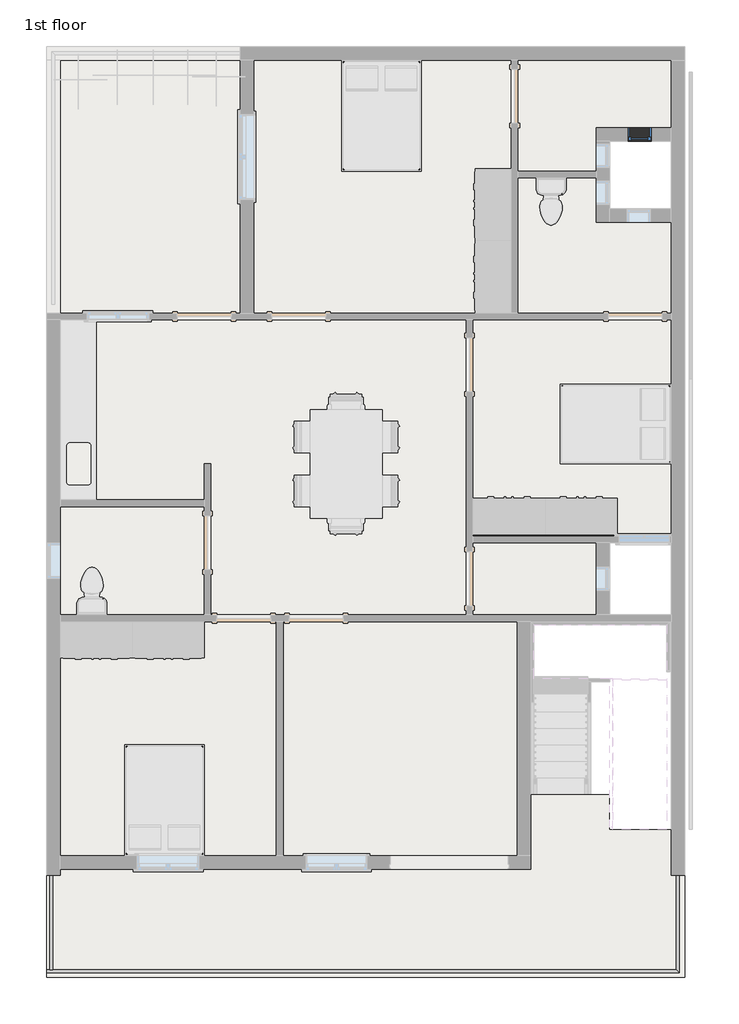
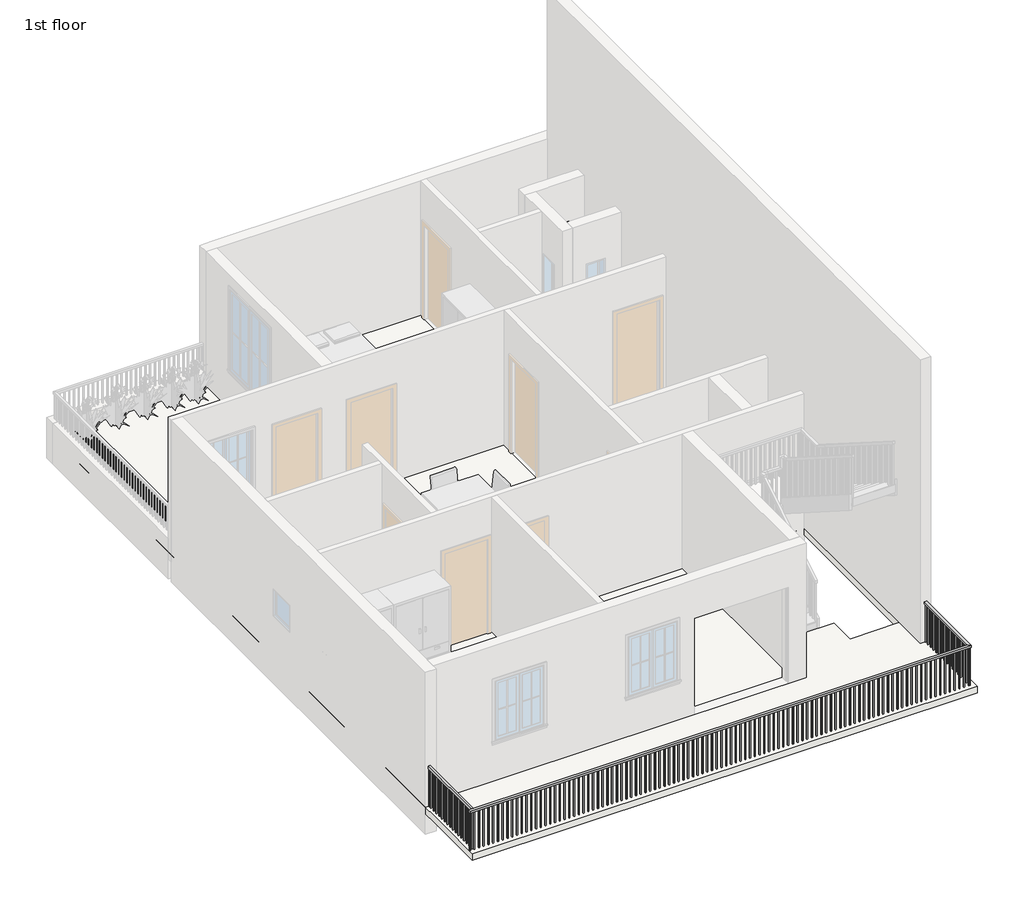
# One storey, part 2 of 5: 2 railings, 1 slab, 1 wall, 1 window.
"""IFC4 building model written with IfcOpenShell, lengths in millimetres."""

from ifc_helpers import new_model, si_unit, frame, origin, place, context, project, spatial, polyline, outline, extrude, faceted_brep, transform, mapped, element, save
from components import window_cea7027f

model = new_model("IFC4")

# Units and contexts
model_context = context("Model", 3, world=origin())
ifc_project = project(units=[si_unit("LENGTHUNIT", "METRE", prefix="MILLI")], contexts=[model_context])

# Site, building, storey
site = spatial("IfcSite", under=ifc_project)
building = spatial("IfcBuilding", under=site)
storey = spatial("IfcBuildingStorey", under=building, Name="1st floor", Elevation=3810.0)

# Railings
placement = place(None, origin())
element("IfcRailing", 1, ObjectType="Handrail - Rectangular", at=placement, inside=storey, context=model_context, shape_type="SolidModel", body=[
    faceted_brep([(-8110.3498597, -2814.1742075, 4724.4), (-8110.3498597, -2814.1742075, 4673.6), (-8110.3498597, -2864.9742075, 4673.6), (-8110.3498597, -2864.9742075, 4724.4), (2544.9501403, -2814.1742075, 4724.4), (2544.9501403, -2814.1742075, 4673.6), (2595.7501403, -2864.9742075, 4673.6), (2595.7501403, -2864.9742075, 4724.4), (2544.9501403, -1213.9742075, 4724.4), (2595.7501403, -1213.9742075, 4724.4), (2595.7501403, -1213.9742075, 4673.6), (2544.9501403, -1213.9742075, 4673.6)], [[[0, 1, 2, 3]], [[1, 0, 4, 5]], [[2, 1, 5, 6]], [[3, 2, 6, 7]], [[0, 3, 7, 4]], [[8, 9, 10, 11]], [[5, 4, 8, 11]], [[6, 5, 11, 10]], [[7, 6, 10, 9]], [[4, 7, 9, 8]]]),
    extrude(outline(polyline([(2579.8751403, -1325.0992075), (2560.8251403, -1325.0992075), (2560.8251403, -1306.0492075), (2579.8751403, -1306.0492075), (2579.8751403, -1325.0992075)])), frame((0.0, 0.0, 3810.0), z_axis=(0.0, 0.0, 1.0), x_axis=(1.0, 0.0, 0.0)), (0.0, 0.0, 1.0), 863.6),
    extrude(outline(polyline([(2579.8751403, -1426.6992075), (2560.8251403, -1426.6992075), (2560.8251403, -1407.6492075), (2579.8751403, -1407.6492075), (2579.8751403, -1426.6992075)])), frame((0.0, 0.0, 3810.0), z_axis=(0.0, 0.0, 1.0), x_axis=(1.0, 0.0, 0.0)), (0.0, 0.0, 1.0), 863.6),
    extrude(outline(polyline([(2579.8751403, -1528.2992075), (2560.8251403, -1528.2992075), (2560.8251403, -1509.2492075), (2579.8751403, -1509.2492075), (2579.8751403, -1528.2992075)])), frame((0.0, 0.0, 3810.0), z_axis=(0.0, 0.0, 1.0), x_axis=(1.0, 0.0, 0.0)), (0.0, 0.0, 1.0), 863.6),
    extrude(outline(polyline([(2579.8751403, -1629.8992075), (2560.8251403, -1629.8992075), (2560.8251403, -1610.8492075), (2579.8751403, -1610.8492075), (2579.8751403, -1629.8992075)])), frame((0.0, 0.0, 3810.0), z_axis=(0.0, 0.0, 1.0), x_axis=(1.0, 0.0, 0.0)), (0.0, 0.0, 1.0), 863.6),
    extrude(outline(polyline([(2579.8751403, -1731.4992075), (2560.8251403, -1731.4992075), (2560.8251403, -1712.4492075), (2579.8751403, -1712.4492075), (2579.8751403, -1731.4992075)])), frame((0.0, 0.0, 3810.0), z_axis=(0.0, 0.0, 1.0), x_axis=(1.0, 0.0, 0.0)), (0.0, 0.0, 1.0), 863.6),
    extrude(outline(polyline([(2579.8751403, -1833.0992075), (2560.8251403, -1833.0992075), (2560.8251403, -1814.0492075), (2579.8751403, -1814.0492075), (2579.8751403, -1833.0992075)])), frame((0.0, 0.0, 3810.0), z_axis=(0.0, 0.0, 1.0), x_axis=(1.0, 0.0, 0.0)), (0.0, 0.0, 1.0), 863.6),
    extrude(outline(polyline([(2579.8751403, -1934.6992075), (2560.8251403, -1934.6992075), (2560.8251403, -1915.6492075), (2579.8751403, -1915.6492075), (2579.8751403, -1934.6992075)])), frame((0.0, 0.0, 3810.0), z_axis=(0.0, 0.0, 1.0), x_axis=(1.0, 0.0, 0.0)), (0.0, 0.0, 1.0), 863.6),
    extrude(outline(polyline([(2579.8751403, -2036.2992075), (2560.8251403, -2036.2992075), (2560.8251403, -2017.2492075), (2579.8751403, -2017.2492075), (2579.8751403, -2036.2992075)])), frame((0.0, 0.0, 3810.0), z_axis=(0.0, 0.0, 1.0), x_axis=(1.0, 0.0, 0.0)), (0.0, 0.0, 1.0), 863.6),
    extrude(outline(polyline([(2579.8751403, -2137.8992075), (2560.8251403, -2137.8992075), (2560.8251403, -2118.8492075), (2579.8751403, -2118.8492075), (2579.8751403, -2137.8992075)])), frame((0.0, 0.0, 3810.0), z_axis=(0.0, 0.0, 1.0), x_axis=(1.0, 0.0, 0.0)), (0.0, 0.0, 1.0), 863.6),
    extrude(outline(polyline([(2579.8751403, -2239.4992075), (2560.8251403, -2239.4992075), (2560.8251403, -2220.4492075), (2579.8751403, -2220.4492075), (2579.8751403, -2239.4992075)])), frame((0.0, 0.0, 3810.0), z_axis=(0.0, 0.0, 1.0), x_axis=(1.0, 0.0, 0.0)), (0.0, 0.0, 1.0), 863.6),
    extrude(outline(polyline([(2579.8751403, -2341.0992075), (2560.8251403, -2341.0992075), (2560.8251403, -2322.0492075), (2579.8751403, -2322.0492075), (2579.8751403, -2341.0992075)])), frame((0.0, 0.0, 3810.0), z_axis=(0.0, 0.0, 1.0), x_axis=(1.0, 0.0, 0.0)), (0.0, 0.0, 1.0), 863.6),
    extrude(outline(polyline([(2579.8751403, -2442.6992075), (2560.8251403, -2442.6992075), (2560.8251403, -2423.6492075), (2579.8751403, -2423.6492075), (2579.8751403, -2442.6992075)])), frame((0.0, 0.0, 3810.0), z_axis=(0.0, 0.0, 1.0), x_axis=(1.0, 0.0, 0.0)), (0.0, 0.0, 1.0), 863.6),
    extrude(outline(polyline([(2579.8751403, -2544.2992075), (2560.8251403, -2544.2992075), (2560.8251403, -2525.2492075), (2579.8751403, -2525.2492075), (2579.8751403, -2544.2992075)])), frame((0.0, 0.0, 3810.0), z_axis=(0.0, 0.0, 1.0), x_axis=(1.0, 0.0, 0.0)), (0.0, 0.0, 1.0), 863.6),
    extrude(outline(polyline([(2579.8751403, -2645.8992075), (2560.8251403, -2645.8992075), (2560.8251403, -2626.8492075), (2579.8751403, -2626.8492075), (2579.8751403, -2645.8992075)])), frame((0.0, 0.0, 3810.0), z_axis=(0.0, 0.0, 1.0), x_axis=(1.0, 0.0, 0.0)), (0.0, 0.0, 1.0), 863.6),
    extrude(outline(polyline([(2579.8751403, -2747.4992075), (2560.8251403, -2747.4992075), (2560.8251403, -2728.4492075), (2579.8751403, -2728.4492075), (2579.8751403, -2747.4992075)])), frame((0.0, 0.0, 3810.0), z_axis=(0.0, 0.0, 1.0), x_axis=(1.0, 0.0, 0.0)), (0.0, 0.0, 1.0), 863.6),
    extrude(outline(polyline([(2548.1251403, -2849.0992075), (2548.1251403, -2830.0492075), (2567.1751403, -2830.0492075), (2567.1751403, -2849.0992075), (2548.1251403, -2849.0992075)])), frame((0.0, 0.0, 3810.0), z_axis=(0.0, 0.0, 1.0), x_axis=(1.0, 0.0, 0.0)), (0.0, 0.0, 1.0), 863.6),
    extrude(outline(polyline([(2446.5251403, -2849.0992075), (2446.5251403, -2830.0492075), (2465.5751403, -2830.0492075), (2465.5751403, -2849.0992075), (2446.5251403, -2849.0992075)])), frame((0.0, 0.0, 3810.0), z_axis=(0.0, 0.0, 1.0), x_axis=(1.0, 0.0, 0.0)), (0.0, 0.0, 1.0), 863.6),
    extrude(outline(polyline([(2344.9251403, -2849.0992075), (2344.9251403, -2830.0492075), (2363.9751403, -2830.0492075), (2363.9751403, -2849.0992075), (2344.9251403, -2849.0992075)])), frame((0.0, 0.0, 3810.0), z_axis=(0.0, 0.0, 1.0), x_axis=(1.0, 0.0, 0.0)), (0.0, 0.0, 1.0), 863.6),
    extrude(outline(polyline([(2243.3251403, -2849.0992075), (2243.3251403, -2830.0492075), (2262.3751403, -2830.0492075), (2262.3751403, -2849.0992075), (2243.3251403, -2849.0992075)])), frame((0.0, 0.0, 3810.0), z_axis=(0.0, 0.0, 1.0), x_axis=(1.0, 0.0, 0.0)), (0.0, 0.0, 1.0), 863.6),
    extrude(outline(polyline([(2141.7251403, -2849.0992075), (2141.7251403, -2830.0492075), (2160.7751403, -2830.0492075), (2160.7751403, -2849.0992075), (2141.7251403, -2849.0992075)])), frame((0.0, 0.0, 3810.0), z_axis=(0.0, 0.0, 1.0), x_axis=(1.0, 0.0, 0.0)), (0.0, 0.0, 1.0), 863.6),
    extrude(outline(polyline([(2040.1251403, -2849.0992075), (2040.1251403, -2830.0492075), (2059.1751403, -2830.0492075), (2059.1751403, -2849.0992075), (2040.1251403, -2849.0992075)])), frame((0.0, 0.0, 3810.0), z_axis=(0.0, 0.0, 1.0), x_axis=(1.0, 0.0, 0.0)), (0.0, 0.0, 1.0), 863.6),
    extrude(outline(polyline([(1938.5251403, -2849.0992075), (1938.5251403, -2830.0492075), (1957.5751403, -2830.0492075), (1957.5751403, -2849.0992075), (1938.5251403, -2849.0992075)])), frame((0.0, 0.0, 3810.0), z_axis=(0.0, 0.0, 1.0), x_axis=(1.0, 0.0, 0.0)), (0.0, 0.0, 1.0), 863.6),
    extrude(outline(polyline([(1836.9251403, -2849.0992075), (1836.9251403, -2830.0492075), (1855.9751403, -2830.0492075), (1855.9751403, -2849.0992075), (1836.9251403, -2849.0992075)])), frame((0.0, 0.0, 3810.0), z_axis=(0.0, 0.0, 1.0), x_axis=(1.0, 0.0, 0.0)), (0.0, 0.0, 1.0), 863.6),
    extrude(outline(polyline([(1735.3251403, -2849.0992075), (1735.3251403, -2830.0492075), (1754.3751403, -2830.0492075), (1754.3751403, -2849.0992075), (1735.3251403, -2849.0992075)])), frame((0.0, 0.0, 3810.0), z_axis=(0.0, 0.0, 1.0), x_axis=(1.0, 0.0, 0.0)), (0.0, 0.0, 1.0), 863.6),
    extrude(outline(polyline([(1633.7251403, -2849.0992075), (1633.7251403, -2830.0492075), (1652.7751403, -2830.0492075), (1652.7751403, -2849.0992075), (1633.7251403, -2849.0992075)])), frame((0.0, 0.0, 3810.0), z_axis=(0.0, 0.0, 1.0), x_axis=(1.0, 0.0, 0.0)), (0.0, 0.0, 1.0), 863.6),
    extrude(outline(polyline([(1532.1251403, -2849.0992075), (1532.1251403, -2830.0492075), (1551.1751403, -2830.0492075), (1551.1751403, -2849.0992075), (1532.1251403, -2849.0992075)])), frame((0.0, 0.0, 3810.0), z_axis=(0.0, 0.0, 1.0), x_axis=(1.0, 0.0, 0.0)), (0.0, 0.0, 1.0), 863.6),
    extrude(outline(polyline([(1430.5251403, -2849.0992075), (1430.5251403, -2830.0492075), (1449.5751403, -2830.0492075), (1449.5751403, -2849.0992075), (1430.5251403, -2849.0992075)])), frame((0.0, 0.0, 3810.0), z_axis=(0.0, 0.0, 1.0), x_axis=(1.0, 0.0, 0.0)), (0.0, 0.0, 1.0), 863.6),
    extrude(outline(polyline([(1328.9251403, -2849.0992075), (1328.9251403, -2830.0492075), (1347.9751403, -2830.0492075), (1347.9751403, -2849.0992075), (1328.9251403, -2849.0992075)])), frame((0.0, 0.0, 3810.0), z_axis=(0.0, 0.0, 1.0), x_axis=(1.0, 0.0, 0.0)), (0.0, 0.0, 1.0), 863.6),
    extrude(outline(polyline([(1227.3251403, -2849.0992075), (1227.3251403, -2830.0492075), (1246.3751403, -2830.0492075), (1246.3751403, -2849.0992075), (1227.3251403, -2849.0992075)])), frame((0.0, 0.0, 3810.0), z_axis=(0.0, 0.0, 1.0), x_axis=(1.0, 0.0, 0.0)), (0.0, 0.0, 1.0), 863.6),
    extrude(outline(polyline([(1125.7251403, -2849.0992075), (1125.7251403, -2830.0492075), (1144.7751403, -2830.0492075), (1144.7751403, -2849.0992075), (1125.7251403, -2849.0992075)])), frame((0.0, 0.0, 3810.0), z_axis=(0.0, 0.0, 1.0), x_axis=(1.0, 0.0, 0.0)), (0.0, 0.0, 1.0), 863.6),
    extrude(outline(polyline([(1024.1251403, -2849.0992075), (1024.1251403, -2830.0492075), (1043.1751403, -2830.0492075), (1043.1751403, -2849.0992075), (1024.1251403, -2849.0992075)])), frame((0.0, 0.0, 3810.0), z_axis=(0.0, 0.0, 1.0), x_axis=(1.0, 0.0, 0.0)), (0.0, 0.0, 1.0), 863.6),
    extrude(outline(polyline([(922.5251403, -2849.0992075), (922.5251403, -2830.0492075), (941.5751403, -2830.0492075), (941.5751403, -2849.0992075), (922.5251403, -2849.0992075)])), frame((0.0, 0.0, 3810.0), z_axis=(0.0, 0.0, 1.0), x_axis=(1.0, 0.0, 0.0)), (0.0, 0.0, 1.0), 863.6),
    extrude(outline(polyline([(820.9251403, -2849.0992075), (820.9251403, -2830.0492075), (839.9751403, -2830.0492075), (839.9751403, -2849.0992075), (820.9251403, -2849.0992075)])), frame((0.0, 0.0, 3810.0), z_axis=(0.0, 0.0, 1.0), x_axis=(1.0, 0.0, 0.0)), (0.0, 0.0, 1.0), 863.6),
    extrude(outline(polyline([(719.3251403, -2849.0992075), (719.3251403, -2830.0492075), (738.3751403, -2830.0492075), (738.3751403, -2849.0992075), (719.3251403, -2849.0992075)])), frame((0.0, 0.0, 3810.0), z_axis=(0.0, 0.0, 1.0), x_axis=(1.0, 0.0, 0.0)), (0.0, 0.0, 1.0), 863.6),
    extrude(outline(polyline([(617.7251403, -2849.0992075), (617.7251403, -2830.0492075), (636.7751403, -2830.0492075), (636.7751403, -2849.0992075), (617.7251403, -2849.0992075)])), frame((0.0, 0.0, 3810.0), z_axis=(0.0, 0.0, 1.0), x_axis=(1.0, 0.0, 0.0)), (0.0, 0.0, 1.0), 863.6),
    extrude(outline(polyline([(516.1251403, -2849.0992075), (516.1251403, -2830.0492075), (535.1751403, -2830.0492075), (535.1751403, -2849.0992075), (516.1251403, -2849.0992075)])), frame((0.0, 0.0, 3810.0), z_axis=(0.0, 0.0, 1.0), x_axis=(1.0, 0.0, 0.0)), (0.0, 0.0, 1.0), 863.6),
    extrude(outline(polyline([(414.5251403, -2849.0992075), (414.5251403, -2830.0492075), (433.5751403, -2830.0492075), (433.5751403, -2849.0992075), (414.5251403, -2849.0992075)])), frame((0.0, 0.0, 3810.0), z_axis=(0.0, 0.0, 1.0), x_axis=(1.0, 0.0, 0.0)), (0.0, 0.0, 1.0), 863.6),
    extrude(outline(polyline([(312.9251403, -2849.0992075), (312.9251403, -2830.0492075), (331.9751403, -2830.0492075), (331.9751403, -2849.0992075), (312.9251403, -2849.0992075)])), frame((0.0, 0.0, 3810.0), z_axis=(0.0, 0.0, 1.0), x_axis=(1.0, 0.0, 0.0)), (0.0, 0.0, 1.0), 863.6),
    extrude(outline(polyline([(211.3251403, -2849.0992075), (211.3251403, -2830.0492075), (230.3751403, -2830.0492075), (230.3751403, -2849.0992075), (211.3251403, -2849.0992075)])), frame((0.0, 0.0, 3810.0), z_axis=(0.0, 0.0, 1.0), x_axis=(1.0, 0.0, 0.0)), (0.0, 0.0, 1.0), 863.6),
    extrude(outline(polyline([(109.7251403, -2849.0992075), (109.7251403, -2830.0492075), (128.7751403, -2830.0492075), (128.7751403, -2849.0992075), (109.7251403, -2849.0992075)])), frame((0.0, 0.0, 3810.0), z_axis=(0.0, 0.0, 1.0), x_axis=(1.0, 0.0, 0.0)), (0.0, 0.0, 1.0), 863.6),
    extrude(outline(polyline([(8.1251403, -2849.0992075), (8.1251403, -2830.0492075), (27.1751403, -2830.0492075), (27.1751403, -2849.0992075), (8.1251403, -2849.0992075)])), frame((0.0, 0.0, 3810.0), z_axis=(0.0, 0.0, 1.0), x_axis=(1.0, 0.0, 0.0)), (0.0, 0.0, 1.0), 863.6),
    extrude(outline(polyline([(-93.4748597, -2849.0992075), (-93.4748597, -2830.0492075), (-74.4248597, -2830.0492075), (-74.4248597, -2849.0992075), (-93.4748597, -2849.0992075)])), frame((0.0, 0.0, 3810.0), z_axis=(0.0, 0.0, 1.0), x_axis=(1.0, 0.0, 0.0)), (0.0, 0.0, 1.0), 863.6),
    extrude(outline(polyline([(-195.0748597, -2849.0992075), (-195.0748597, -2830.0492075), (-176.0248597, -2830.0492075), (-176.0248597, -2849.0992075), (-195.0748597, -2849.0992075)])), frame((0.0, 0.0, 3810.0), z_axis=(0.0, 0.0, 1.0), x_axis=(1.0, 0.0, 0.0)), (0.0, 0.0, 1.0), 863.6),
    extrude(outline(polyline([(-296.6748597, -2849.0992075), (-296.6748597, -2830.0492075), (-277.6248597, -2830.0492075), (-277.6248597, -2849.0992075), (-296.6748597, -2849.0992075)])), frame((0.0, 0.0, 3810.0), z_axis=(0.0, 0.0, 1.0), x_axis=(1.0, 0.0, 0.0)), (0.0, 0.0, 1.0), 863.6),
    extrude(outline(polyline([(-398.2748597, -2849.0992075), (-398.2748597, -2830.0492075), (-379.2248597, -2830.0492075), (-379.2248597, -2849.0992075), (-398.2748597, -2849.0992075)])), frame((0.0, 0.0, 3810.0), z_axis=(0.0, 0.0, 1.0), x_axis=(1.0, 0.0, 0.0)), (0.0, 0.0, 1.0), 863.6),
    extrude(outline(polyline([(-499.8748597, -2849.0992075), (-499.8748597, -2830.0492075), (-480.8248597, -2830.0492075), (-480.8248597, -2849.0992075), (-499.8748597, -2849.0992075)])), frame((0.0, 0.0, 3810.0), z_axis=(0.0, 0.0, 1.0), x_axis=(1.0, 0.0, 0.0)), (0.0, 0.0, 1.0), 863.6),
    extrude(outline(polyline([(-601.4748597, -2849.0992075), (-601.4748597, -2830.0492075), (-582.4248597, -2830.0492075), (-582.4248597, -2849.0992075), (-601.4748597, -2849.0992075)])), frame((0.0, 0.0, 3810.0), z_axis=(0.0, 0.0, 1.0), x_axis=(1.0, 0.0, 0.0)), (0.0, 0.0, 1.0), 863.6),
    extrude(outline(polyline([(-703.0748597, -2849.0992075), (-703.0748597, -2830.0492075), (-684.0248597, -2830.0492075), (-684.0248597, -2849.0992075), (-703.0748597, -2849.0992075)])), frame((0.0, 0.0, 3810.0), z_axis=(0.0, 0.0, 1.0), x_axis=(1.0, 0.0, 0.0)), (0.0, 0.0, 1.0), 863.6),
    extrude(outline(polyline([(-804.6748597, -2849.0992075), (-804.6748597, -2830.0492075), (-785.6248597, -2830.0492075), (-785.6248597, -2849.0992075), (-804.6748597, -2849.0992075)])), frame((0.0, 0.0, 3810.0), z_axis=(0.0, 0.0, 1.0), x_axis=(1.0, 0.0, 0.0)), (0.0, 0.0, 1.0), 863.6),
    extrude(outline(polyline([(-906.2748597, -2849.0992075), (-906.2748597, -2830.0492075), (-887.2248597, -2830.0492075), (-887.2248597, -2849.0992075), (-906.2748597, -2849.0992075)])), frame((0.0, 0.0, 3810.0), z_axis=(0.0, 0.0, 1.0), x_axis=(1.0, 0.0, 0.0)), (0.0, 0.0, 1.0), 863.6),
    extrude(outline(polyline([(-1007.8748597, -2849.0992075), (-1007.8748597, -2830.0492075), (-988.8248597, -2830.0492075), (-988.8248597, -2849.0992075), (-1007.8748597, -2849.0992075)])), frame((0.0, 0.0, 3810.0), z_axis=(0.0, 0.0, 1.0), x_axis=(1.0, 0.0, 0.0)), (0.0, 0.0, 1.0), 863.6),
    extrude(outline(polyline([(-1109.4748597, -2849.0992075), (-1109.4748597, -2830.0492075), (-1090.4248597, -2830.0492075), (-1090.4248597, -2849.0992075), (-1109.4748597, -2849.0992075)])), frame((0.0, 0.0, 3810.0), z_axis=(0.0, 0.0, 1.0), x_axis=(1.0, 0.0, 0.0)), (0.0, 0.0, 1.0), 863.6),
    extrude(outline(polyline([(-1211.0748597, -2849.0992075), (-1211.0748597, -2830.0492075), (-1192.0248597, -2830.0492075), (-1192.0248597, -2849.0992075), (-1211.0748597, -2849.0992075)])), frame((0.0, 0.0, 3810.0), z_axis=(0.0, 0.0, 1.0), x_axis=(1.0, 0.0, 0.0)), (0.0, 0.0, 1.0), 863.6),
    extrude(outline(polyline([(-1312.6748597, -2849.0992075), (-1312.6748597, -2830.0492075), (-1293.6248597, -2830.0492075), (-1293.6248597, -2849.0992075), (-1312.6748597, -2849.0992075)])), frame((0.0, 0.0, 3810.0), z_axis=(0.0, 0.0, 1.0), x_axis=(1.0, 0.0, 0.0)), (0.0, 0.0, 1.0), 863.6),
    extrude(outline(polyline([(-1414.2748597, -2849.0992075), (-1414.2748597, -2830.0492075), (-1395.2248597, -2830.0492075), (-1395.2248597, -2849.0992075), (-1414.2748597, -2849.0992075)])), frame((0.0, 0.0, 3810.0), z_axis=(0.0, 0.0, 1.0), x_axis=(1.0, 0.0, 0.0)), (0.0, 0.0, 1.0), 863.6),
    extrude(outline(polyline([(-1515.8748597, -2849.0992075), (-1515.8748597, -2830.0492075), (-1496.8248597, -2830.0492075), (-1496.8248597, -2849.0992075), (-1515.8748597, -2849.0992075)])), frame((0.0, 0.0, 3810.0), z_axis=(0.0, 0.0, 1.0), x_axis=(1.0, 0.0, 0.0)), (0.0, 0.0, 1.0), 863.6),
    extrude(outline(polyline([(-1617.4748597, -2849.0992075), (-1617.4748597, -2830.0492075), (-1598.4248597, -2830.0492075), (-1598.4248597, -2849.0992075), (-1617.4748597, -2849.0992075)])), frame((0.0, 0.0, 3810.0), z_axis=(0.0, 0.0, 1.0), x_axis=(1.0, 0.0, 0.0)), (0.0, 0.0, 1.0), 863.6),
    extrude(outline(polyline([(-1719.0748597, -2849.0992075), (-1719.0748597, -2830.0492075), (-1700.0248597, -2830.0492075), (-1700.0248597, -2849.0992075), (-1719.0748597, -2849.0992075)])), frame((0.0, 0.0, 3810.0), z_axis=(0.0, 0.0, 1.0), x_axis=(1.0, 0.0, 0.0)), (0.0, 0.0, 1.0), 863.6),
    extrude(outline(polyline([(-1820.6748597, -2849.0992075), (-1820.6748597, -2830.0492075), (-1801.6248597, -2830.0492075), (-1801.6248597, -2849.0992075), (-1820.6748597, -2849.0992075)])), frame((0.0, 0.0, 3810.0), z_axis=(0.0, 0.0, 1.0), x_axis=(1.0, 0.0, 0.0)), (0.0, 0.0, 1.0), 863.6),
    extrude(outline(polyline([(-1922.2748597, -2849.0992075), (-1922.2748597, -2830.0492075), (-1903.2248597, -2830.0492075), (-1903.2248597, -2849.0992075), (-1922.2748597, -2849.0992075)])), frame((0.0, 0.0, 3810.0), z_axis=(0.0, 0.0, 1.0), x_axis=(1.0, 0.0, 0.0)), (0.0, 0.0, 1.0), 863.6),
    extrude(outline(polyline([(-2023.8748597, -2849.0992075), (-2023.8748597, -2830.0492075), (-2004.8248597, -2830.0492075), (-2004.8248597, -2849.0992075), (-2023.8748597, -2849.0992075)])), frame((0.0, 0.0, 3810.0), z_axis=(0.0, 0.0, 1.0), x_axis=(1.0, 0.0, 0.0)), (0.0, 0.0, 1.0), 863.6),
    extrude(outline(polyline([(-2125.4748597, -2849.0992075), (-2125.4748597, -2830.0492075), (-2106.4248597, -2830.0492075), (-2106.4248597, -2849.0992075), (-2125.4748597, -2849.0992075)])), frame((0.0, 0.0, 3810.0), z_axis=(0.0, 0.0, 1.0), x_axis=(1.0, 0.0, 0.0)), (0.0, 0.0, 1.0), 863.6),
    extrude(outline(polyline([(-2227.0748597, -2849.0992075), (-2227.0748597, -2830.0492075), (-2208.0248597, -2830.0492075), (-2208.0248597, -2849.0992075), (-2227.0748597, -2849.0992075)])), frame((0.0, 0.0, 3810.0), z_axis=(0.0, 0.0, 1.0), x_axis=(1.0, 0.0, 0.0)), (0.0, 0.0, 1.0), 863.6),
    extrude(outline(polyline([(-2328.6748597, -2849.0992075), (-2328.6748597, -2830.0492075), (-2309.6248597, -2830.0492075), (-2309.6248597, -2849.0992075), (-2328.6748597, -2849.0992075)])), frame((0.0, 0.0, 3810.0), z_axis=(0.0, 0.0, 1.0), x_axis=(1.0, 0.0, 0.0)), (0.0, 0.0, 1.0), 863.6),
    extrude(outline(polyline([(-2430.2748597, -2849.0992075), (-2430.2748597, -2830.0492075), (-2411.2248597, -2830.0492075), (-2411.2248597, -2849.0992075), (-2430.2748597, -2849.0992075)])), frame((0.0, 0.0, 3810.0), z_axis=(0.0, 0.0, 1.0), x_axis=(1.0, 0.0, 0.0)), (0.0, 0.0, 1.0), 863.6),
    extrude(outline(polyline([(-2531.8748597, -2849.0992075), (-2531.8748597, -2830.0492075), (-2512.8248597, -2830.0492075), (-2512.8248597, -2849.0992075), (-2531.8748597, -2849.0992075)])), frame((0.0, 0.0, 3810.0), z_axis=(0.0, 0.0, 1.0), x_axis=(1.0, 0.0, 0.0)), (0.0, 0.0, 1.0), 863.6),
    extrude(outline(polyline([(-2633.4748597, -2849.0992075), (-2633.4748597, -2830.0492075), (-2614.4248597, -2830.0492075), (-2614.4248597, -2849.0992075), (-2633.4748597, -2849.0992075)])), frame((0.0, 0.0, 3810.0), z_axis=(0.0, 0.0, 1.0), x_axis=(1.0, 0.0, 0.0)), (0.0, 0.0, 1.0), 863.6),
    extrude(outline(polyline([(-2735.0748597, -2849.0992075), (-2735.0748597, -2830.0492075), (-2716.0248597, -2830.0492075), (-2716.0248597, -2849.0992075), (-2735.0748597, -2849.0992075)])), frame((0.0, 0.0, 3810.0), z_axis=(0.0, 0.0, 1.0), x_axis=(1.0, 0.0, 0.0)), (0.0, 0.0, 1.0), 863.6),
    extrude(outline(polyline([(-2836.6748597, -2849.0992075), (-2836.6748597, -2830.0492075), (-2817.6248597, -2830.0492075), (-2817.6248597, -2849.0992075), (-2836.6748597, -2849.0992075)])), frame((0.0, 0.0, 3810.0), z_axis=(0.0, 0.0, 1.0), x_axis=(1.0, 0.0, 0.0)), (0.0, 0.0, 1.0), 863.6),
    extrude(outline(polyline([(-2938.2748597, -2849.0992075), (-2938.2748597, -2830.0492075), (-2919.2248597, -2830.0492075), (-2919.2248597, -2849.0992075), (-2938.2748597, -2849.0992075)])), frame((0.0, 0.0, 3810.0), z_axis=(0.0, 0.0, 1.0), x_axis=(1.0, 0.0, 0.0)), (0.0, 0.0, 1.0), 863.6),
    extrude(outline(polyline([(-3039.8748597, -2849.0992075), (-3039.8748597, -2830.0492075), (-3020.8248597, -2830.0492075), (-3020.8248597, -2849.0992075), (-3039.8748597, -2849.0992075)])), frame((0.0, 0.0, 3810.0), z_axis=(0.0, 0.0, 1.0), x_axis=(1.0, 0.0, 0.0)), (0.0, 0.0, 1.0), 863.6),
    extrude(outline(polyline([(-3141.4748597, -2849.0992075), (-3141.4748597, -2830.0492075), (-3122.4248597, -2830.0492075), (-3122.4248597, -2849.0992075), (-3141.4748597, -2849.0992075)])), frame((0.0, 0.0, 3810.0), z_axis=(0.0, 0.0, 1.0), x_axis=(1.0, 0.0, 0.0)), (0.0, 0.0, 1.0), 863.6),
    extrude(outline(polyline([(-3243.0748597, -2849.0992075), (-3243.0748597, -2830.0492075), (-3224.0248597, -2830.0492075), (-3224.0248597, -2849.0992075), (-3243.0748597, -2849.0992075)])), frame((0.0, 0.0, 3810.0), z_axis=(0.0, 0.0, 1.0), x_axis=(1.0, 0.0, 0.0)), (0.0, 0.0, 1.0), 863.6),
    extrude(outline(polyline([(-3344.6748597, -2849.0992075), (-3344.6748597, -2830.0492075), (-3325.6248597, -2830.0492075), (-3325.6248597, -2849.0992075), (-3344.6748597, -2849.0992075)])), frame((0.0, 0.0, 3810.0), z_axis=(0.0, 0.0, 1.0), x_axis=(1.0, 0.0, 0.0)), (0.0, 0.0, 1.0), 863.6),
    extrude(outline(polyline([(-3446.2748597, -2849.0992075), (-3446.2748597, -2830.0492075), (-3427.2248597, -2830.0492075), (-3427.2248597, -2849.0992075), (-3446.2748597, -2849.0992075)])), frame((0.0, 0.0, 3810.0), z_axis=(0.0, 0.0, 1.0), x_axis=(1.0, 0.0, 0.0)), (0.0, 0.0, 1.0), 863.6),
    extrude(outline(polyline([(-3547.8748597, -2849.0992075), (-3547.8748597, -2830.0492075), (-3528.8248597, -2830.0492075), (-3528.8248597, -2849.0992075), (-3547.8748597, -2849.0992075)])), frame((0.0, 0.0, 3810.0), z_axis=(0.0, 0.0, 1.0), x_axis=(1.0, 0.0, 0.0)), (0.0, 0.0, 1.0), 863.6),
    extrude(outline(polyline([(-3649.4748597, -2849.0992075), (-3649.4748597, -2830.0492075), (-3630.4248597, -2830.0492075), (-3630.4248597, -2849.0992075), (-3649.4748597, -2849.0992075)])), frame((0.0, 0.0, 3810.0), z_axis=(0.0, 0.0, 1.0), x_axis=(1.0, 0.0, 0.0)), (0.0, 0.0, 1.0), 863.6),
    extrude(outline(polyline([(-3751.0748597, -2849.0992075), (-3751.0748597, -2830.0492075), (-3732.0248597, -2830.0492075), (-3732.0248597, -2849.0992075), (-3751.0748597, -2849.0992075)])), frame((0.0, 0.0, 3810.0), z_axis=(0.0, 0.0, 1.0), x_axis=(1.0, 0.0, 0.0)), (0.0, 0.0, 1.0), 863.6),
    extrude(outline(polyline([(-3852.6748597, -2849.0992075), (-3852.6748597, -2830.0492075), (-3833.6248597, -2830.0492075), (-3833.6248597, -2849.0992075), (-3852.6748597, -2849.0992075)])), frame((0.0, 0.0, 3810.0), z_axis=(0.0, 0.0, 1.0), x_axis=(1.0, 0.0, 0.0)), (0.0, 0.0, 1.0), 863.6),
    extrude(outline(polyline([(-3954.2748597, -2849.0992075), (-3954.2748597, -2830.0492075), (-3935.2248597, -2830.0492075), (-3935.2248597, -2849.0992075), (-3954.2748597, -2849.0992075)])), frame((0.0, 0.0, 3810.0), z_axis=(0.0, 0.0, 1.0), x_axis=(1.0, 0.0, 0.0)), (0.0, 0.0, 1.0), 863.6),
    extrude(outline(polyline([(-4055.8748597, -2849.0992075), (-4055.8748597, -2830.0492075), (-4036.8248597, -2830.0492075), (-4036.8248597, -2849.0992075), (-4055.8748597, -2849.0992075)])), frame((0.0, 0.0, 3810.0), z_axis=(0.0, 0.0, 1.0), x_axis=(1.0, 0.0, 0.0)), (0.0, 0.0, 1.0), 863.6),
    extrude(outline(polyline([(-4157.4748597, -2849.0992075), (-4157.4748597, -2830.0492075), (-4138.4248597, -2830.0492075), (-4138.4248597, -2849.0992075), (-4157.4748597, -2849.0992075)])), frame((0.0, 0.0, 3810.0), z_axis=(0.0, 0.0, 1.0), x_axis=(1.0, 0.0, 0.0)), (0.0, 0.0, 1.0), 863.6),
    extrude(outline(polyline([(-4259.0748597, -2849.0992075), (-4259.0748597, -2830.0492075), (-4240.0248597, -2830.0492075), (-4240.0248597, -2849.0992075), (-4259.0748597, -2849.0992075)])), frame((0.0, 0.0, 3810.0), z_axis=(0.0, 0.0, 1.0), x_axis=(1.0, 0.0, 0.0)), (0.0, 0.0, 1.0), 863.6),
    extrude(outline(polyline([(-4360.6748597, -2849.0992075), (-4360.6748597, -2830.0492075), (-4341.6248597, -2830.0492075), (-4341.6248597, -2849.0992075), (-4360.6748597, -2849.0992075)])), frame((0.0, 0.0, 3810.0), z_axis=(0.0, 0.0, 1.0), x_axis=(1.0, 0.0, 0.0)), (0.0, 0.0, 1.0), 863.6),
    extrude(outline(polyline([(-4462.2748597, -2849.0992075), (-4462.2748597, -2830.0492075), (-4443.2248597, -2830.0492075), (-4443.2248597, -2849.0992075), (-4462.2748597, -2849.0992075)])), frame((0.0, 0.0, 3810.0), z_axis=(0.0, 0.0, 1.0), x_axis=(1.0, 0.0, 0.0)), (0.0, 0.0, 1.0), 863.6),
    extrude(outline(polyline([(-4563.8748597, -2849.0992075), (-4563.8748597, -2830.0492075), (-4544.8248597, -2830.0492075), (-4544.8248597, -2849.0992075), (-4563.8748597, -2849.0992075)])), frame((0.0, 0.0, 3810.0), z_axis=(0.0, 0.0, 1.0), x_axis=(1.0, 0.0, 0.0)), (0.0, 0.0, 1.0), 863.6),
    extrude(outline(polyline([(-4665.4748597, -2849.0992075), (-4665.4748597, -2830.0492075), (-4646.4248597, -2830.0492075), (-4646.4248597, -2849.0992075), (-4665.4748597, -2849.0992075)])), frame((0.0, 0.0, 3810.0), z_axis=(0.0, 0.0, 1.0), x_axis=(1.0, 0.0, 0.0)), (0.0, 0.0, 1.0), 863.6),
    extrude(outline(polyline([(-4767.0748597, -2849.0992075), (-4767.0748597, -2830.0492075), (-4748.0248597, -2830.0492075), (-4748.0248597, -2849.0992075), (-4767.0748597, -2849.0992075)])), frame((0.0, 0.0, 3810.0), z_axis=(0.0, 0.0, 1.0), x_axis=(1.0, 0.0, 0.0)), (0.0, 0.0, 1.0), 863.6),
    extrude(outline(polyline([(-4868.6748597, -2849.0992075), (-4868.6748597, -2830.0492075), (-4849.6248597, -2830.0492075), (-4849.6248597, -2849.0992075), (-4868.6748597, -2849.0992075)])), frame((0.0, 0.0, 3810.0), z_axis=(0.0, 0.0, 1.0), x_axis=(1.0, 0.0, 0.0)), (0.0, 0.0, 1.0), 863.6),
    extrude(outline(polyline([(-4970.2748597, -2849.0992075), (-4970.2748597, -2830.0492075), (-4951.2248597, -2830.0492075), (-4951.2248597, -2849.0992075), (-4970.2748597, -2849.0992075)])), frame((0.0, 0.0, 3810.0), z_axis=(0.0, 0.0, 1.0), x_axis=(1.0, 0.0, 0.0)), (0.0, 0.0, 1.0), 863.6),
    extrude(outline(polyline([(-5071.8748597, -2849.0992075), (-5071.8748597, -2830.0492075), (-5052.8248597, -2830.0492075), (-5052.8248597, -2849.0992075), (-5071.8748597, -2849.0992075)])), frame((0.0, 0.0, 3810.0), z_axis=(0.0, 0.0, 1.0), x_axis=(1.0, 0.0, 0.0)), (0.0, 0.0, 1.0), 863.6),
    extrude(outline(polyline([(-5173.4748597, -2849.0992075), (-5173.4748597, -2830.0492075), (-5154.4248597, -2830.0492075), (-5154.4248597, -2849.0992075), (-5173.4748597, -2849.0992075)])), frame((0.0, 0.0, 3810.0), z_axis=(0.0, 0.0, 1.0), x_axis=(1.0, 0.0, 0.0)), (0.0, 0.0, 1.0), 863.6),
    extrude(outline(polyline([(-5275.0748597, -2849.0992075), (-5275.0748597, -2830.0492075), (-5256.0248597, -2830.0492075), (-5256.0248597, -2849.0992075), (-5275.0748597, -2849.0992075)])), frame((0.0, 0.0, 3810.0), z_axis=(0.0, 0.0, 1.0), x_axis=(1.0, 0.0, 0.0)), (0.0, 0.0, 1.0), 863.6),
    extrude(outline(polyline([(-5376.6748597, -2849.0992075), (-5376.6748597, -2830.0492075), (-5357.6248597, -2830.0492075), (-5357.6248597, -2849.0992075), (-5376.6748597, -2849.0992075)])), frame((0.0, 0.0, 3810.0), z_axis=(0.0, 0.0, 1.0), x_axis=(1.0, 0.0, 0.0)), (0.0, 0.0, 1.0), 863.6),
    extrude(outline(polyline([(-5478.2748597, -2849.0992075), (-5478.2748597, -2830.0492075), (-5459.2248597, -2830.0492075), (-5459.2248597, -2849.0992075), (-5478.2748597, -2849.0992075)])), frame((0.0, 0.0, 3810.0), z_axis=(0.0, 0.0, 1.0), x_axis=(1.0, 0.0, 0.0)), (0.0, 0.0, 1.0), 863.6),
    extrude(outline(polyline([(-5579.8748597, -2849.0992075), (-5579.8748597, -2830.0492075), (-5560.8248597, -2830.0492075), (-5560.8248597, -2849.0992075), (-5579.8748597, -2849.0992075)])), frame((0.0, 0.0, 3810.0), z_axis=(0.0, 0.0, 1.0), x_axis=(1.0, 0.0, 0.0)), (0.0, 0.0, 1.0), 863.6),
    extrude(outline(polyline([(-5681.4748597, -2849.0992075), (-5681.4748597, -2830.0492075), (-5662.4248597, -2830.0492075), (-5662.4248597, -2849.0992075), (-5681.4748597, -2849.0992075)])), frame((0.0, 0.0, 3810.0), z_axis=(0.0, 0.0, 1.0), x_axis=(1.0, 0.0, 0.0)), (0.0, 0.0, 1.0), 863.6),
    extrude(outline(polyline([(-5783.0748597, -2849.0992075), (-5783.0748597, -2830.0492075), (-5764.0248597, -2830.0492075), (-5764.0248597, -2849.0992075), (-5783.0748597, -2849.0992075)])), frame((0.0, 0.0, 3810.0), z_axis=(0.0, 0.0, 1.0), x_axis=(1.0, 0.0, 0.0)), (0.0, 0.0, 1.0), 863.6),
    extrude(outline(polyline([(-5884.6748597, -2849.0992075), (-5884.6748597, -2830.0492075), (-5865.6248597, -2830.0492075), (-5865.6248597, -2849.0992075), (-5884.6748597, -2849.0992075)])), frame((0.0, 0.0, 3810.0), z_axis=(0.0, 0.0, 1.0), x_axis=(1.0, 0.0, 0.0)), (0.0, 0.0, 1.0), 863.6),
    extrude(outline(polyline([(-5986.2748597, -2849.0992075), (-5986.2748597, -2830.0492075), (-5967.2248597, -2830.0492075), (-5967.2248597, -2849.0992075), (-5986.2748597, -2849.0992075)])), frame((0.0, 0.0, 3810.0), z_axis=(0.0, 0.0, 1.0), x_axis=(1.0, 0.0, 0.0)), (0.0, 0.0, 1.0), 863.6),
    extrude(outline(polyline([(-6087.8748597, -2849.0992075), (-6087.8748597, -2830.0492075), (-6068.8248597, -2830.0492075), (-6068.8248597, -2849.0992075), (-6087.8748597, -2849.0992075)])), frame((0.0, 0.0, 3810.0), z_axis=(0.0, 0.0, 1.0), x_axis=(1.0, 0.0, 0.0)), (0.0, 0.0, 1.0), 863.6),
    extrude(outline(polyline([(-6189.4748597, -2849.0992075), (-6189.4748597, -2830.0492075), (-6170.4248597, -2830.0492075), (-6170.4248597, -2849.0992075), (-6189.4748597, -2849.0992075)])), frame((0.0, 0.0, 3810.0), z_axis=(0.0, 0.0, 1.0), x_axis=(1.0, 0.0, 0.0)), (0.0, 0.0, 1.0), 863.6),
    extrude(outline(polyline([(-6291.0748597, -2849.0992075), (-6291.0748597, -2830.0492075), (-6272.0248597, -2830.0492075), (-6272.0248597, -2849.0992075), (-6291.0748597, -2849.0992075)])), frame((0.0, 0.0, 3810.0), z_axis=(0.0, 0.0, 1.0), x_axis=(1.0, 0.0, 0.0)), (0.0, 0.0, 1.0), 863.6),
    extrude(outline(polyline([(-6392.6748597, -2849.0992075), (-6392.6748597, -2830.0492075), (-6373.6248597, -2830.0492075), (-6373.6248597, -2849.0992075), (-6392.6748597, -2849.0992075)])), frame((0.0, 0.0, 3810.0), z_axis=(0.0, 0.0, 1.0), x_axis=(1.0, 0.0, 0.0)), (0.0, 0.0, 1.0), 863.6),
    extrude(outline(polyline([(-6494.2748597, -2849.0992075), (-6494.2748597, -2830.0492075), (-6475.2248597, -2830.0492075), (-6475.2248597, -2849.0992075), (-6494.2748597, -2849.0992075)])), frame((0.0, 0.0, 3810.0), z_axis=(0.0, 0.0, 1.0), x_axis=(1.0, 0.0, 0.0)), (0.0, 0.0, 1.0), 863.6),
    extrude(outline(polyline([(-6595.8748597, -2849.0992075), (-6595.8748597, -2830.0492075), (-6576.8248597, -2830.0492075), (-6576.8248597, -2849.0992075), (-6595.8748597, -2849.0992075)])), frame((0.0, 0.0, 3810.0), z_axis=(0.0, 0.0, 1.0), x_axis=(1.0, 0.0, 0.0)), (0.0, 0.0, 1.0), 863.6),
    extrude(outline(polyline([(-6697.4748597, -2849.0992075), (-6697.4748597, -2830.0492075), (-6678.4248597, -2830.0492075), (-6678.4248597, -2849.0992075), (-6697.4748597, -2849.0992075)])), frame((0.0, 0.0, 3810.0), z_axis=(0.0, 0.0, 1.0), x_axis=(1.0, 0.0, 0.0)), (0.0, 0.0, 1.0), 863.6),
    extrude(outline(polyline([(-6799.0748597, -2849.0992075), (-6799.0748597, -2830.0492075), (-6780.0248597, -2830.0492075), (-6780.0248597, -2849.0992075), (-6799.0748597, -2849.0992075)])), frame((0.0, 0.0, 3810.0), z_axis=(0.0, 0.0, 1.0), x_axis=(1.0, 0.0, 0.0)), (0.0, 0.0, 1.0), 863.6),
    extrude(outline(polyline([(-6900.6748597, -2849.0992075), (-6900.6748597, -2830.0492075), (-6881.6248597, -2830.0492075), (-6881.6248597, -2849.0992075), (-6900.6748597, -2849.0992075)])), frame((0.0, 0.0, 3810.0), z_axis=(0.0, 0.0, 1.0), x_axis=(1.0, 0.0, 0.0)), (0.0, 0.0, 1.0), 863.6),
    extrude(outline(polyline([(-7002.2748597, -2849.0992075), (-7002.2748597, -2830.0492075), (-6983.2248597, -2830.0492075), (-6983.2248597, -2849.0992075), (-7002.2748597, -2849.0992075)])), frame((0.0, 0.0, 3810.0), z_axis=(0.0, 0.0, 1.0), x_axis=(1.0, 0.0, 0.0)), (0.0, 0.0, 1.0), 863.6),
    extrude(outline(polyline([(-7103.8748597, -2849.0992075), (-7103.8748597, -2830.0492075), (-7084.8248597, -2830.0492075), (-7084.8248597, -2849.0992075), (-7103.8748597, -2849.0992075)])), frame((0.0, 0.0, 3810.0), z_axis=(0.0, 0.0, 1.0), x_axis=(1.0, 0.0, 0.0)), (0.0, 0.0, 1.0), 863.6),
    extrude(outline(polyline([(-7205.4748597, -2849.0992075), (-7205.4748597, -2830.0492075), (-7186.4248597, -2830.0492075), (-7186.4248597, -2849.0992075), (-7205.4748597, -2849.0992075)])), frame((0.0, 0.0, 3810.0), z_axis=(0.0, 0.0, 1.0), x_axis=(1.0, 0.0, 0.0)), (0.0, 0.0, 1.0), 863.6),
    extrude(outline(polyline([(-7307.0748597, -2849.0992075), (-7307.0748597, -2830.0492075), (-7288.0248597, -2830.0492075), (-7288.0248597, -2849.0992075), (-7307.0748597, -2849.0992075)])), frame((0.0, 0.0, 3810.0), z_axis=(0.0, 0.0, 1.0), x_axis=(1.0, 0.0, 0.0)), (0.0, 0.0, 1.0), 863.6),
    extrude(outline(polyline([(-7408.6748597, -2849.0992075), (-7408.6748597, -2830.0492075), (-7389.6248597, -2830.0492075), (-7389.6248597, -2849.0992075), (-7408.6748597, -2849.0992075)])), frame((0.0, 0.0, 3810.0), z_axis=(0.0, 0.0, 1.0), x_axis=(1.0, 0.0, 0.0)), (0.0, 0.0, 1.0), 863.6),
    extrude(outline(polyline([(-7510.2748597, -2849.0992075), (-7510.2748597, -2830.0492075), (-7491.2248597, -2830.0492075), (-7491.2248597, -2849.0992075), (-7510.2748597, -2849.0992075)])), frame((0.0, 0.0, 3810.0), z_axis=(0.0, 0.0, 1.0), x_axis=(1.0, 0.0, 0.0)), (0.0, 0.0, 1.0), 863.6),
    extrude(outline(polyline([(-7611.8748597, -2849.0992075), (-7611.8748597, -2830.0492075), (-7592.8248597, -2830.0492075), (-7592.8248597, -2849.0992075), (-7611.8748597, -2849.0992075)])), frame((0.0, 0.0, 3810.0), z_axis=(0.0, 0.0, 1.0), x_axis=(1.0, 0.0, 0.0)), (0.0, 0.0, 1.0), 863.6),
    extrude(outline(polyline([(-7713.4748597, -2849.0992075), (-7713.4748597, -2830.0492075), (-7694.4248597, -2830.0492075), (-7694.4248597, -2849.0992075), (-7713.4748597, -2849.0992075)])), frame((0.0, 0.0, 3810.0), z_axis=(0.0, 0.0, 1.0), x_axis=(1.0, 0.0, 0.0)), (0.0, 0.0, 1.0), 863.6),
    extrude(outline(polyline([(-7815.0748597, -2849.0992075), (-7815.0748597, -2830.0492075), (-7796.0248597, -2830.0492075), (-7796.0248597, -2849.0992075), (-7815.0748597, -2849.0992075)])), frame((0.0, 0.0, 3810.0), z_axis=(0.0, 0.0, 1.0), x_axis=(1.0, 0.0, 0.0)), (0.0, 0.0, 1.0), 863.6),
    extrude(outline(polyline([(-7916.6748597, -2849.0992075), (-7916.6748597, -2830.0492075), (-7897.6248597, -2830.0492075), (-7897.6248597, -2849.0992075), (-7916.6748597, -2849.0992075)])), frame((0.0, 0.0, 3810.0), z_axis=(0.0, 0.0, 1.0), x_axis=(1.0, 0.0, 0.0)), (0.0, 0.0, 1.0), 863.6),
    extrude(outline(polyline([(-8018.2748597, -2849.0992075), (-8018.2748597, -2830.0492075), (-7999.2248597, -2830.0492075), (-7999.2248597, -2849.0992075), (-8018.2748597, -2849.0992075)])), frame((0.0, 0.0, 3810.0), z_axis=(0.0, 0.0, 1.0), x_axis=(1.0, 0.0, 0.0)), (0.0, 0.0, 1.0), 863.6),
    extrude(outline(polyline([(2560.8251403, -2849.0992075), (2560.8251403, -2830.0492075), (2579.8751403, -2830.0492075), (2579.8751403, -2849.0992075), (2560.8251403, -2849.0992075)])), frame((0.0, 0.0, 3810.0), z_axis=(0.0, 0.0, 1.0), x_axis=(1.0, 0.0, 0.0)), (0.0, 0.0, 1.0), 863.6),
    extrude(outline(polyline([(2579.8751403, -1233.0242075), (2560.8251403, -1233.0242075), (2560.8251403, -1213.9742075), (2579.8751403, -1213.9742075), (2579.8751403, -1233.0242075)])), frame((0.0, 0.0, 3810.0), z_axis=(0.0, 0.0, 1.0), x_axis=(1.0, 0.0, 0.0)), (0.0, 0.0, 1.0), 863.6),
    extrude(outline(polyline([(-8110.3498597, -2849.0992075), (-8110.3498597, -2830.0492075), (-8091.2998597, -2830.0492075), (-8091.2998597, -2849.0992075), (-8110.3498597, -2849.0992075)])), frame((0.0, 0.0, 3810.0), z_axis=(0.0, 0.0, 1.0), x_axis=(1.0, 0.0, 0.0)), (0.0, 0.0, 1.0), 863.6),
])
element("IfcRailing", 2, ObjectType="Handrail - Rectangular", at=placement, inside=storey, context=model_context, shape_type="SweptSolid", body=[
    extrude(outline(polyline([(-8008.7498597, -2814.1742075), (-8059.5498597, -2814.1742075), (-8059.5498597, -1213.9742075), (-8008.7498597, -1213.9742075), (-8008.7498597, -2814.1742075)])), frame((0.0, 0.0, 4673.6), z_axis=(0.0, 0.0, 1.0), x_axis=(1.0, 0.0, 0.0)), (0.0, 0.0, 1.0), 50.8),
    extrude(outline(polyline([(-8024.6248597, -1299.6992075), (-8043.6748597, -1299.6992075), (-8043.6748597, -1280.6492075), (-8024.6248597, -1280.6492075), (-8024.6248597, -1299.6992075)])), frame((0.0, 0.0, 3810.0), z_axis=(0.0, 0.0, 1.0), x_axis=(1.0, 0.0, 0.0)), (0.0, 0.0, 1.0), 863.6),
    extrude(outline(polyline([(-8024.6248597, -1401.2992075), (-8043.6748597, -1401.2992075), (-8043.6748597, -1382.2492075), (-8024.6248597, -1382.2492075), (-8024.6248597, -1401.2992075)])), frame((0.0, 0.0, 3810.0), z_axis=(0.0, 0.0, 1.0), x_axis=(1.0, 0.0, 0.0)), (0.0, 0.0, 1.0), 863.6),
    extrude(outline(polyline([(-8024.6248597, -1502.8992075), (-8043.6748597, -1502.8992075), (-8043.6748597, -1483.8492075), (-8024.6248597, -1483.8492075), (-8024.6248597, -1502.8992075)])), frame((0.0, 0.0, 3810.0), z_axis=(0.0, 0.0, 1.0), x_axis=(1.0, 0.0, 0.0)), (0.0, 0.0, 1.0), 863.6),
    extrude(outline(polyline([(-8024.6248597, -1604.4992075), (-8043.6748597, -1604.4992075), (-8043.6748597, -1585.4492075), (-8024.6248597, -1585.4492075), (-8024.6248597, -1604.4992075)])), frame((0.0, 0.0, 3810.0), z_axis=(0.0, 0.0, 1.0), x_axis=(1.0, 0.0, 0.0)), (0.0, 0.0, 1.0), 863.6),
    extrude(outline(polyline([(-8024.6248597, -1706.0992075), (-8043.6748597, -1706.0992075), (-8043.6748597, -1687.0492075), (-8024.6248597, -1687.0492075), (-8024.6248597, -1706.0992075)])), frame((0.0, 0.0, 3810.0), z_axis=(0.0, 0.0, 1.0), x_axis=(1.0, 0.0, 0.0)), (0.0, 0.0, 1.0), 863.6),
    extrude(outline(polyline([(-8024.6248597, -1807.6992075), (-8043.6748597, -1807.6992075), (-8043.6748597, -1788.6492075), (-8024.6248597, -1788.6492075), (-8024.6248597, -1807.6992075)])), frame((0.0, 0.0, 3810.0), z_axis=(0.0, 0.0, 1.0), x_axis=(1.0, 0.0, 0.0)), (0.0, 0.0, 1.0), 863.6),
    extrude(outline(polyline([(-8024.6248597, -1909.2992075), (-8043.6748597, -1909.2992075), (-8043.6748597, -1890.2492075), (-8024.6248597, -1890.2492075), (-8024.6248597, -1909.2992075)])), frame((0.0, 0.0, 3810.0), z_axis=(0.0, 0.0, 1.0), x_axis=(1.0, 0.0, 0.0)), (0.0, 0.0, 1.0), 863.6),
    extrude(outline(polyline([(-8024.6248597, -2010.8992075), (-8043.6748597, -2010.8992075), (-8043.6748597, -1991.8492075), (-8024.6248597, -1991.8492075), (-8024.6248597, -2010.8992075)])), frame((0.0, 0.0, 3810.0), z_axis=(0.0, 0.0, 1.0), x_axis=(1.0, 0.0, 0.0)), (0.0, 0.0, 1.0), 863.6),
    extrude(outline(polyline([(-8024.6248597, -2112.4992075), (-8043.6748597, -2112.4992075), (-8043.6748597, -2093.4492075), (-8024.6248597, -2093.4492075), (-8024.6248597, -2112.4992075)])), frame((0.0, 0.0, 3810.0), z_axis=(0.0, 0.0, 1.0), x_axis=(1.0, 0.0, 0.0)), (0.0, 0.0, 1.0), 863.6),
    extrude(outline(polyline([(-8024.6248597, -2214.0992075), (-8043.6748597, -2214.0992075), (-8043.6748597, -2195.0492075), (-8024.6248597, -2195.0492075), (-8024.6248597, -2214.0992075)])), frame((0.0, 0.0, 3810.0), z_axis=(0.0, 0.0, 1.0), x_axis=(1.0, 0.0, 0.0)), (0.0, 0.0, 1.0), 863.6),
    extrude(outline(polyline([(-8024.6248597, -2315.6992075), (-8043.6748597, -2315.6992075), (-8043.6748597, -2296.6492075), (-8024.6248597, -2296.6492075), (-8024.6248597, -2315.6992075)])), frame((0.0, 0.0, 3810.0), z_axis=(0.0, 0.0, 1.0), x_axis=(1.0, 0.0, 0.0)), (0.0, 0.0, 1.0), 863.6),
    extrude(outline(polyline([(-8024.6248597, -2417.2992075), (-8043.6748597, -2417.2992075), (-8043.6748597, -2398.2492075), (-8024.6248597, -2398.2492075), (-8024.6248597, -2417.2992075)])), frame((0.0, 0.0, 3810.0), z_axis=(0.0, 0.0, 1.0), x_axis=(1.0, 0.0, 0.0)), (0.0, 0.0, 1.0), 863.6),
    extrude(outline(polyline([(-8024.6248597, -2518.8992075), (-8043.6748597, -2518.8992075), (-8043.6748597, -2499.8492075), (-8024.6248597, -2499.8492075), (-8024.6248597, -2518.8992075)])), frame((0.0, 0.0, 3810.0), z_axis=(0.0, 0.0, 1.0), x_axis=(1.0, 0.0, 0.0)), (0.0, 0.0, 1.0), 863.6),
    extrude(outline(polyline([(-8024.6248597, -2620.4992075), (-8043.6748597, -2620.4992075), (-8043.6748597, -2601.4492075), (-8024.6248597, -2601.4492075), (-8024.6248597, -2620.4992075)])), frame((0.0, 0.0, 3810.0), z_axis=(0.0, 0.0, 1.0), x_axis=(1.0, 0.0, 0.0)), (0.0, 0.0, 1.0), 863.6),
    extrude(outline(polyline([(-8024.6248597, -2722.0992075), (-8043.6748597, -2722.0992075), (-8043.6748597, -2703.0492075), (-8024.6248597, -2703.0492075), (-8024.6248597, -2722.0992075)])), frame((0.0, 0.0, 3810.0), z_axis=(0.0, 0.0, 1.0), x_axis=(1.0, 0.0, 0.0)), (0.0, 0.0, 1.0), 863.6),
    extrude(outline(polyline([(-8024.6248597, -1233.0242075), (-8043.6748597, -1233.0242075), (-8043.6748597, -1213.9742075), (-8024.6248597, -1213.9742075), (-8024.6248597, -1233.0242075)])), frame((0.0, 0.0, 3810.0), z_axis=(0.0, 0.0, 1.0), x_axis=(1.0, 0.0, 0.0)), (0.0, 0.0, 1.0), 863.6),
    extrude(outline(polyline([(-8024.6248597, -2814.1742075), (-8043.6748597, -2814.1742075), (-8043.6748597, -2795.1242075), (-8024.6248597, -2795.1242075), (-8024.6248597, -2814.1742075)])), frame((0.0, 0.0, 3810.0), z_axis=(0.0, 0.0, 1.0), x_axis=(1.0, 0.0, 0.0)), (0.0, 0.0, 1.0), 863.6),
])

# Slab
element("IfcSlab", 3, at=placement, inside=storey, context=model_context, shape_type="SweptSolid", body=[
    extrude(outline(polyline([(2684.6501403, 12806.8257925), (2684.6501403, -2941.1742075), (-8110.3498597, -2941.1742075), (-8110.3498597, 12806.8257925), (2684.6501403, 12806.8257925)]), holes=[polyline([(81.1501403, 3078.6257925), (81.1501403, 157.6257925), (1414.6501403, 157.6257925), (1414.6501403, -432.9242075), (2456.0501403, -432.9242075), (2456.0501403, 3078.6257925), (2430.6501403, 3078.6257925), (81.1501403, 3078.6257925)]), polyline([(2456.0501403, 11206.6257925), (1414.6501403, 11206.6257925), (1414.6501403, 10063.6257925), (2456.0501403, 10063.6257925), (2456.0501403, 11206.6257925)]), polyline([(2456.0501403, 4412.1257925), (1414.6501403, 4412.1257925), (1414.6501403, 3192.9257925), (2456.0501403, 3192.9257925), (2456.0501403, 4412.1257925)])]), frame((0.0, 0.0, 3657.6), z_axis=(0.0, 0.0, 1.0), x_axis=(1.0, 0.0, 0.0)), (0.0, 0.0, 1.0), 152.4),
])

# Wall
element("IfcWall", 4, at=placement, inside=storey, context=model_context, shape_type="SweptSolid", body=[
    extrude(outline(polyline([(1414.6501403, 11435.2257925), (2456.0501403, 11435.2257925), (2456.0501403, 11206.6257925), (1414.6501403, 11206.6257925), (1414.6501403, 11435.2257925)])), frame((0.0, 0.0, 3200.4), z_axis=(0.0, 0.0, 1.0), x_axis=(1.0, 0.0, 0.0)), (0.0, 0.0, 1.0), 3657.6),
])

# Window
window_shape = window_cea7027f(model_context)
element("IfcWindow", 5, ObjectType="Fixed : 16\" x 48\"", at=placement, inside=storey, context=model_context, shape_type="MappedRepresentation", body=[
    mapped(window_shape, transform((1884.5501403, 11320.9257925, 3810.0), x_axis=(-1.0, 0.0, 0.0), y_axis=(0.0, -1.0, 0.0), z_axis=(0.0, 0.0, 1.0))),
])

save(model, "model.ifc")

# Revit data of these elements
# Type "Handrail - Rectangular"
#   Assembly Code = "C2010400"
#   built-in parameter 1008612 = 0.0416667 (stored number, unit not read)
#   built-in parameter 1008611 = 0.0416667 (stored number, unit not read)
#   built-in parameter 1008609 = 0.333333 (stored number, unit not read)
#   built-in parameter 1008604 = 0.166667 (stored number, unit not read)
#   built-in parameter 1008603 = 0.166667 (stored number, unit not read)
#   Railing Height = 3' - 0"
#   built-in parameter 1008630 = 2
#   built-in parameter 1008610 = 2
#   built-in parameter 1008618 = Baluster - Square : 3/4"
# Type
#   Assembly Code = "B1010"
#   Function = 0
#   Layers, outside or top first: 0' - 6" "Concrete, Cast-in-Place gray" (function 1)
# Type
#   Assembly Code = "B2010"
#   Layers, outside or top first: 0' - 9" no material (function 1)
# Type "Fixed : 16\" x 48\""
#   Type Mark = "5"
#   Construction Type Id = "GSP4R"
#   Assembly Code = "B2020100"
#   Analytic Construction = "1/8 in Pilkington single glazing"
#   Visual Light Transmittance = 0.9
#   Solar Heat Gain Coefficient = 0.78
#   Heat Transfer Coefficient (U) = 0.6496 BTU/(h·ft²·°F)
#   Height = 4' - 0"
#   Default Sill Height = 3' - 0"
#   Width = 1' - 4"
#   Window Inset = 0' - 0 3/4"
#   Define Thermal Properties by = 1
#   Define Thermal Properties by = 1
#   Glass Pane Material = Glass
#   Sash Material = Sash
#   Wall Closure = (empty or 0)
# Elements 1, 2 (IfcRailing, "Handrail - Rectangular")
#   Phase Created = New Construction
# Element 3 (IfcSlab)
#   Height Offset From Level = 0' - 0"
#   Phase Created = New Construction
#   Materials on its faces: "Concrete, Cast-in-Place gray"
# Element 4 (IfcWall)
#   built-in parameter 1001111 = -2' - 0"
#   Top Offset = 0' - 0"
#   Base Offset = -2' - 0"
#   wall height = 12' - 0"
#   Phase Created = New Construction
#   Base Constraint = 1st floor
#   Top Constraint = 2nd floor
#   Materials on its faces: "Default Wall"
# Element 5 (IfcWindow, "Fixed : 16\" x 48\"")
#   Mark = "20"
#   Phase Created = New Construction
#   Materials on its faces: "Sash", "Glass"
# Materials
#   "Concrete, Cast-in-Place gray": class "Concrete", colour RGB 192 192 192, transparency 0, Description = "Cast-in-place concrete", Cost = 0
#   "Glass": class "Glass", colour RGB 0 128 192, transparency 0.75, Description = "Soda Lime Glass", Cost = 0
#   "Sash": class "Wood", colour RGB 224 178 126, transparency 0, Cost = 0
#   "Default Wall": colour RGB 128 128 128, transparency 0, Cost = 0
